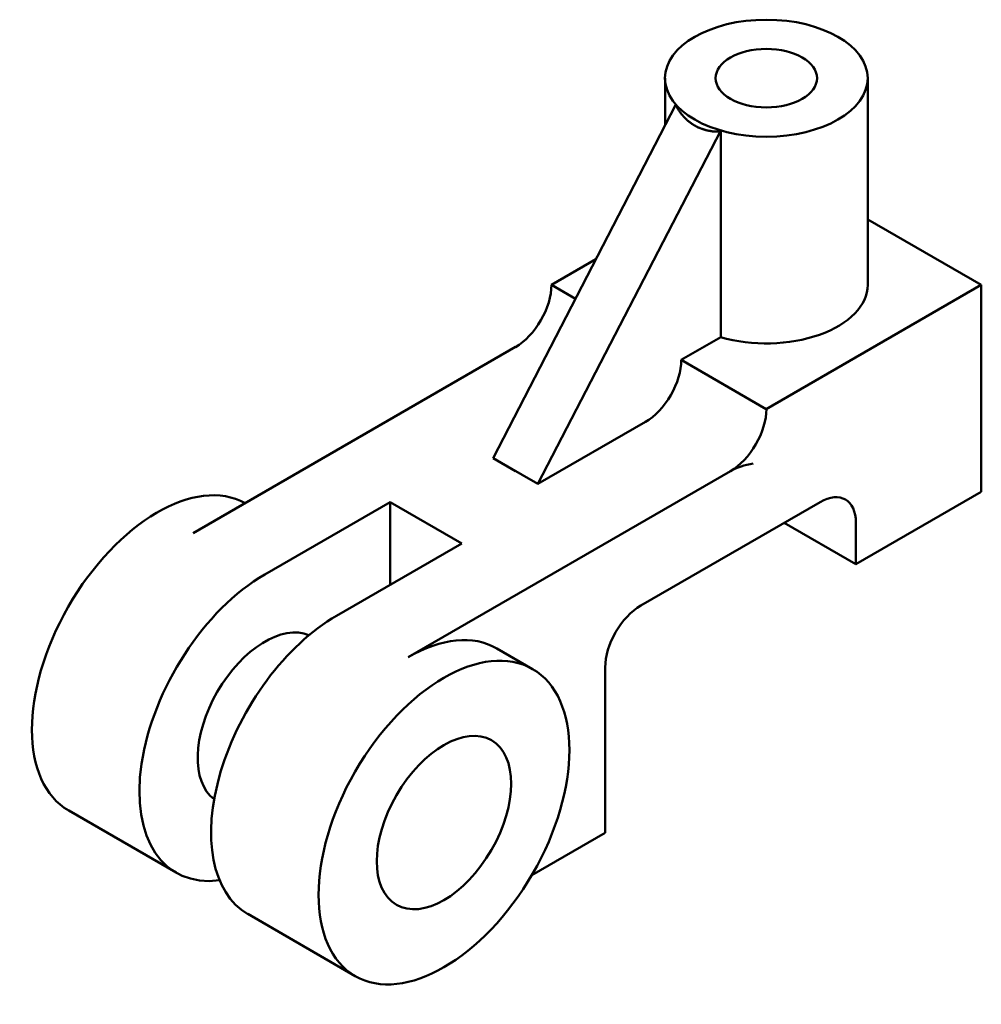
# Model space of a CAD drawing. Units: millimetres. Extents: x 3075 to 3261, y 1554 to 1744.
import ezdxf

# ---------------------------------------------------------------- set-up
doc = ezdxf.new("R2010")
doc.units = ezdxf.units.MM
doc.layers.add('M-OUTL', color=7, linetype='Continuous', lineweight=50)

msp = doc.modelspace()

# ---------------------------------------------------------------- linework, layer by layer
at = {"layer": 'M-OUTL'}
for p, q in [((3199.45, 1732.91), (3199.45, 1723.74)), ((3238.64, 1732.91), (3238.64, 1692.91)), ((3201.55, 1727.82), (3166.22, 1659.41)), ((3174.88, 1654.41), (3210.21, 1722.82)), ((3210.21, 1682.82), (3210.21, 1722.82)), ((3260.61, 1692.91), (3238.64, 1705.6)), ((3186.09, 1697.89), (3177.48, 1692.91)), ((3177.48, 1692.91), (3182.13, 1690.23)), ((3260.61, 1692.91), (3219.04, 1668.91)), ((3260.61, 1652.91), (3260.61, 1692.91)), ((3202.59, 1678.41), (3210.21, 1682.82)), ((3108.19, 1644.91), (3170.55, 1680.91)), ((3219.04, 1668.91), (3202.59, 1678.41)), ((3174.88, 1654.41), (3195.66, 1666.41)), ((3170.55, 1656.91), (3166.22, 1659.41)), ((3166.22, 1659.41), (3174.88, 1654.41)), ((3212.12, 1656.91), (3149.76, 1620.91)), ((3236.37, 1638.91), (3260.61, 1652.91)), ((3146.3, 1650.91), (3122.05, 1636.91)), ((3160.16, 1642.91), (3146.3, 1650.91)), ((3146.3, 1650.91), (3146.3, 1634.91)), ((3229.44, 1650.91), (3194.8, 1630.91)), ((3236.37, 1638.91), (3222.51, 1646.91)), ((3236.37, 1638.91), (3236.37, 1646.91)), ((3135.91, 1628.91), (3160.16, 1642.91)), ((3166.91, 1622.61), (3173.84, 1618.61)), ((3187.87, 1618.91), (3187.87, 1586.91)), ((3104.9, 1579.22), (3084.12, 1591.22)), ((3187.87, 1586.91), (3173.66, 1578.71)), ((3139.54, 1559.22), (3118.76, 1571.22))]:
    msp.add_line(p, q, dxfattribs=at)
msp.add_lwpolyline([(3210.21, 1722.58), (3210.1, 1722.58), (3209.98, 1722.58), (3209.87, 1722.58), (3209.75, 1722.58), (3209.64, 1722.58), (3209.53, 1722.58), (3209.41, 1722.58), (3209.3, 1722.59), (3209.19, 1722.59), (3209.08, 1722.6), (3208.97, 1722.61), (3208.85, 1722.62), (3208.74, 1722.62), (3208.63, 1722.63), (3208.52, 1722.65), (3208.41, 1722.67), (3208.31, 1722.68), (3208.2, 1722.7), (3208.09, 1722.71), (3207.98, 1722.73), (3207.87, 1722.75), (3207.77, 1722.77), (3207.66, 1722.8), (3207.56, 1722.82), (3207.45, 1722.85), (3207.35, 1722.87), (3207.24, 1722.89), (3207.14, 1722.92), (3207.04, 1722.96), (3206.94, 1722.99), (3206.84, 1723.02), (3206.73, 1723.05), (3206.63, 1723.09), (3206.53, 1723.12), (3206.43, 1723.16), (3206.33, 1723.2), (3206.24, 1723.24), (3206.14, 1723.28), (3206.04, 1723.32), (3205.94, 1723.36), (3205.85, 1723.4), (3205.75, 1723.45), (3205.66, 1723.5), (3205.56, 1723.55), (3205.47, 1723.6), (3205.38, 1723.65), (3205.28, 1723.69), (3205.19, 1723.74), (3205.1, 1723.8), (3205.01, 1723.86), (3204.92, 1723.91), (3204.83, 1723.97), (3204.74, 1724.03), (3204.65, 1724.09), (3204.56, 1724.14), (3204.48, 1724.21), (3204.39, 1724.27), (3204.31, 1724.34), (3204.22, 1724.4), (3204.14, 1724.47), (3204.05, 1724.53), (3203.97, 1724.6), (3203.89, 1724.67), (3203.8, 1724.74), (3203.72, 1724.82), (3203.64, 1724.89), (3203.56, 1724.96), (3203.48, 1725.04), (3203.4, 1725.11), (3203.33, 1725.19), (3203.25, 1725.27), (3203.17, 1725.35), (3203.1, 1725.43), (3203.02, 1725.51), (3202.95, 1725.59), (3202.87, 1725.68), (3202.8, 1725.77), (3202.73, 1725.85), (3202.66, 1725.94), (3202.59, 1726.03), (3202.52, 1726.12), (3202.45, 1726.2), (3202.38, 1726.3), (3202.31, 1726.39), (3202.25, 1726.49), (3202.18, 1726.58), (3202.11, 1726.68), (3202.05, 1726.77), (3201.98, 1726.87), (3201.92, 1726.97), (3201.86, 1727.07), (3201.8, 1727.17), (3201.74, 1727.28), (3201.67, 1727.38), (3201.61, 1727.48), (3201.55, 1727.58)], dxfattribs=at)
for centre, major_axis in [((3219.04, 1732.91), (-19.6, 0)), ((3219.04, 1732.91), (-9.8, 0)), ((3156.69, 1588.91), (-17.15, -29.7)), ((3156.69, 1588.91), (-9.19, -15.91))]:
    msp.add_ellipse(centre, major_axis=major_axis, ratio=0.57735, dxfattribs=at)
for centre, major_axis, start_param, end_param in [((3170.55, 1688.91), (-4.9, -8.49), 7.068583, 8.63938), ((3219.04, 1692.91), (-19.6, 0), 1.103222, 3.141593), ((3195.66, 1674.41), (-4.9, -8.49), 7.068583, 8.63938), ((3212.12, 1664.91), (-4.9, -8.49), 7.068583, 8.63938), ((3219.05, 1652.91), (9.8, 0), 1.832596, 2.356194), ((3101.27, 1620.91), (-17.15, -29.7), 3.151797, 6.283185), ((3122.05, 1608.91), (-17.15, -29.7), 3.926991, 6.699137), ((3194.8, 1622.91), (-4.9, -8.49), 3.926991, 5.497787), ((3135.91, 1600.91), (-17.15, -29.7), 3.926991, 6.283185), ((3135.91, 1600.91), (-17.15, -29.7), 3.926991, 6.283185), ((3122.05, 1608.91), (-9.19, -15.91), 3.210886, 6.213892), ((3149.76, 1592.91), (-17.15, -29.7), 3.141593, 3.926991)]:
    msp.add_ellipse(centre, major_axis=major_axis, ratio=0.57735, start_param=start_param, end_param=end_param, dxfattribs=at)
at = {"layer": 'M-OUTL', "extrusion": (0, 0, -1)}
msp.add_ellipse((3229.44, 1642.91), major_axis=(4.9, 8.49), ratio=0.57735, start_param=5.497787, end_param=7.068583, dxfattribs=at)

doc.saveas('drawing.dxf')
